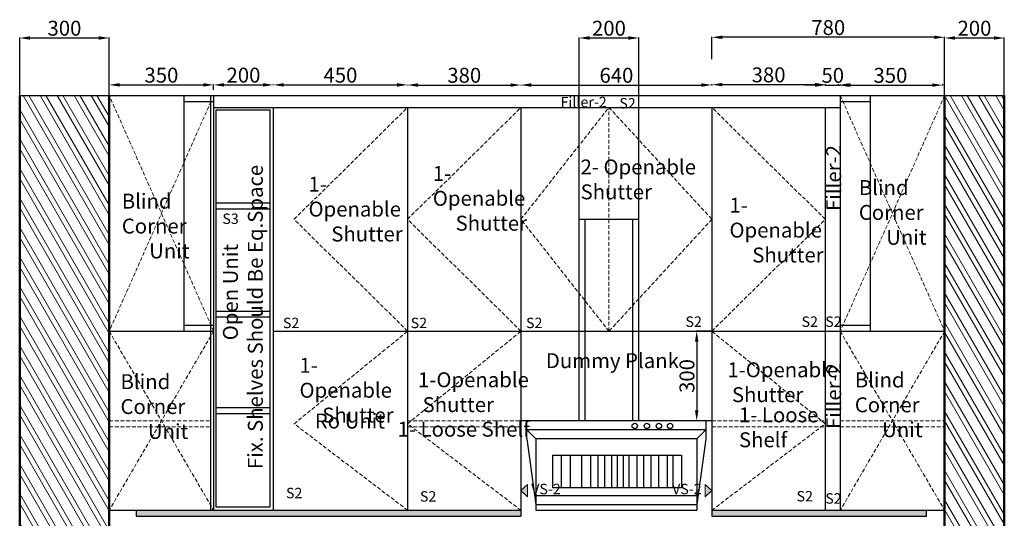
# Model space of a CAD drawing. Units: millimetres. Extents: x 407065 to 421840, y 1168257 to 1177792.
# Tile 13 of 17: x 412429 to 415729, y 1175560 to 1177230. Entities that reach past the tile are written whole.
import ezdxf

# ---------------------------------------------------------------- set-up
doc = ezdxf.new("R2010")
doc.units = ezdxf.units.MM
doc.linetypes.add('DASHED', pattern=[19.05, 12.7, -6.35])
for name, color, linetype, lineweight in [('A-ANNO-DIMS', 6, 'Continuous', 18), ('A-ANNO-SYMB', 6, 'Continuous', 18), ('A-ANNO-TEXT', 30, 'Continuous', 18), ('A-FURN', 3, 'Continuous', 25), ('A-FURN-HIDN', 7, 'DASHED', 18), ('A-FURN-PATT', 252, 'Continuous', 13), ('A-WALL', 7, 'Continuous', 50), ('A-WALL-PATT', 8, 'Continuous', 13)]:
    doc.layers.add(name, color=color, linetype=linetype, lineweight=lineweight)
doc.styles.get("Standard").update_dxf_attribs({"font": 'arial.ttf'})
doc.dimstyles.new('ISO-25', dxfattribs={"dimtxt": 50, "dimasz": 35, "dimexe": 1.25, "dimexo": 0.625, "dimtad": 1, "dimdec": 1, "dimtxsty": 'Standard', "dimcen": 35, "dimadec": 0, "dimazin": 0, "dimtfac": 1, "dimtdec": 1, "dimtmove": 0, "dimatfit": 3, "dimfxl": 1, "dimarcsym": 0})
pattern_1 = [(120, (-2714.86, -161.38), (-42.8942382, -24.765), []), (120, (-2708.816, -138.83), (-42.8942382, -24.765), [])]

# ---------------------------------------------------------------- blocks, each defined once
blk = doc.blocks.new('*D54')
at = {"layer": 'A-ANNO-DIMS', "color": 0, "lineweight": -2, "transparency": 16777216}
for p, q in [((412728.5, 1176995.6), (412728.5, 1177013)), ((412763.5, 1177011.8), (413043.5, 1177011.8)), ((413078.5, 1176995.6), (413078.5, 1177013))]:
    blk.add_line(p, q, dxfattribs=at)
at = {"layer": 'A-ANNO-DIMS', "color": 0, "transparency": 16777216}
for points in [[(412763.5, 1177017.6), (412763.5, 1177005.9), (412728.5, 1177011.8)], [(413043.5, 1177017.6), (413043.5, 1177005.9), (413078.5, 1177011.8)]]:
    blk.add_solid(points, dxfattribs=at)
at = {"layer": 'Defpoints', "color": 0, "transparency": 16777216}
for p in [(413078.5, 1177011.8), (412728.5, 1176995), (413078.5, 1176995)]:
    blk.add_point(p, dxfattribs=at)
at = {"layer": 'A-ANNO-DIMS', "color": 0, "transparency": 16777216, "insert": (412903.5, 1177037.9), "char_height": 50, "attachment_point": 5}
blk.add_mtext('350', dxfattribs=at)
blk = doc.blocks.new('*D55')
at = {"layer": 'A-ANNO-DIMS', "color": 0, "lineweight": -2, "transparency": 16777216}
for p, q in [((413078.5, 1177012.4), (413078.5, 1177013)), ((413113.5, 1177011.8), (413243.5, 1177011.8)), ((413278.5, 1177012.4), (413278.5, 1177013))]:
    blk.add_line(p, q, dxfattribs=at)
at = {"layer": 'A-ANNO-DIMS', "color": 0, "transparency": 16777216}
for points in [[(413113.5, 1177017.6), (413113.5, 1177005.9), (413078.5, 1177011.8)], [(413243.5, 1177017.6), (413243.5, 1177005.9), (413278.5, 1177011.8)]]:
    blk.add_solid(points, dxfattribs=at)
at = {"layer": 'Defpoints', "color": 0, "transparency": 16777216}
for p in [(413078.5, 1177011.8), (413278.5, 1177011.8), (413278.5, 1177011.8)]:
    blk.add_point(p, dxfattribs=at)
at = {"layer": 'A-ANNO-DIMS', "color": 0, "transparency": 16777216, "insert": (413178.5, 1177037.9), "char_height": 50, "attachment_point": 5}
blk.add_mtext('200', dxfattribs=at)
blk = doc.blocks.new('*D56')
at = {"layer": 'A-ANNO-DIMS', "color": 0, "lineweight": -2, "transparency": 16777216}
for p, q in [((413278.5, 1177012.1), (413278.5, 1177010.5)), ((413313.5, 1177011.8), (413693.5, 1177011.8)), ((413728.5, 1177012.1), (413728.5, 1177010.5))]:
    blk.add_line(p, q, dxfattribs=at)
at = {"layer": 'A-ANNO-DIMS', "color": 0, "transparency": 16777216}
for points in [[(413313.5, 1177017.6), (413313.5, 1177005.9), (413278.5, 1177011.8)], [(413693.5, 1177017.6), (413693.5, 1177005.9), (413728.5, 1177011.8)]]:
    blk.add_solid(points, dxfattribs=at)
at = {"layer": 'Defpoints', "color": 0, "transparency": 16777216}
for p in [(413278.5, 1177012.7), (413728.5, 1177012.7), (413728.5, 1177011.8)]:
    blk.add_point(p, dxfattribs=at)
at = {"layer": 'A-ANNO-DIMS', "color": 0, "transparency": 16777216, "insert": (413503.5, 1177037.9), "char_height": 50, "attachment_point": 5}
blk.add_mtext('450', dxfattribs=at)
blk = doc.blocks.new('*D57')
at = {"layer": 'A-ANNO-DIMS', "color": 0, "lineweight": -2, "transparency": 16777216}
for p, q in [((413728.5, 1177012.1), (413728.5, 1177010)), ((413763.5, 1177011.3), (414073.5, 1177011.3)), ((414108.5, 1177012.1), (414108.5, 1177010))]:
    blk.add_line(p, q, dxfattribs=at)
at = {"layer": 'A-ANNO-DIMS', "color": 0, "transparency": 16777216}
for points in [[(413763.5, 1177017.1), (413763.5, 1177005.4), (413728.5, 1177011.3)], [(414073.5, 1177017.1), (414073.5, 1177005.4), (414108.5, 1177011.3)]]:
    blk.add_solid(points, dxfattribs=at)
at = {"layer": 'Defpoints', "color": 0, "transparency": 16777216}
for p in [(413728.5, 1177012.7), (414108.5, 1177012.7), (414108.5, 1177011.3)]:
    blk.add_point(p, dxfattribs=at)
at = {"layer": 'A-ANNO-DIMS', "color": 0, "transparency": 16777216, "insert": (413918.5, 1177037.5), "char_height": 50, "attachment_point": 5}
blk.add_mtext('380', dxfattribs=at)
blk = doc.blocks.new('*D58')
at = {"layer": 'A-ANNO-DIMS', "color": 0, "lineweight": -2, "transparency": 16777216}
for p, q in [((414108.5, 1177012.1), (414108.5, 1177010)), ((414143.5, 1177011.3), (414713.5, 1177011.3)), ((414748.5, 1177012.1), (414748.5, 1177010))]:
    blk.add_line(p, q, dxfattribs=at)
at = {"layer": 'A-ANNO-DIMS', "color": 0, "transparency": 16777216}
for points in [[(414143.5, 1177017.1), (414143.5, 1177005.4), (414108.5, 1177011.3)], [(414713.5, 1177017.1), (414713.5, 1177005.4), (414748.5, 1177011.3)]]:
    blk.add_solid(points, dxfattribs=at)
at = {"layer": 'Defpoints', "color": 0, "transparency": 16777216}
for p in [(414108.5, 1177012.7), (414748.5, 1177012.7), (414748.5, 1177011.3)]:
    blk.add_point(p, dxfattribs=at)
at = {"layer": 'A-ANNO-DIMS', "color": 0, "transparency": 16777216, "insert": (414428.5, 1177037.4), "char_height": 50, "attachment_point": 5}
blk.add_mtext('640', dxfattribs=at)
blk = doc.blocks.new('*D59')
at = {"layer": 'A-ANNO-DIMS', "color": 0, "lineweight": -2, "transparency": 16777216}
for p, q in [((414748.5, 1177011.7), (414748.5, 1177013.9)), ((414783.5, 1177012.7), (415093.5, 1177012.7)), ((415128.5, 1177011.7), (415128.5, 1177013.9))]:
    blk.add_line(p, q, dxfattribs=at)
at = {"layer": 'A-ANNO-DIMS', "color": 0, "transparency": 16777216}
for points in [[(414783.5, 1177018.5), (414783.5, 1177006.9), (414748.5, 1177012.7)], [(415093.5, 1177018.5), (415093.5, 1177006.9), (415128.5, 1177012.7)]]:
    blk.add_solid(points, dxfattribs=at)
at = {"layer": 'Defpoints', "color": 0, "transparency": 16777216}
for p in [(414748.5, 1177011), (415128.5, 1177012.7), (415128.5, 1177011)]:
    blk.add_point(p, dxfattribs=at)
at = {"layer": 'A-ANNO-DIMS', "color": 0, "transparency": 16777216, "insert": (414938.5, 1177038.9), "char_height": 50, "attachment_point": 5}
blk.add_mtext('380', dxfattribs=at)
blk = doc.blocks.new('*D60')
at = {"layer": 'A-ANNO-DIMS', "color": 0, "lineweight": -2, "transparency": 16777216}
for p, q in [((415093.5, 1177011), (415058.5, 1177011)), ((415128.5, 1177013.3), (415128.5, 1177009.8)), ((415128.5, 1177011), (415178.5, 1177011)), ((415178.5, 1177013.3), (415178.5, 1177009.8)), ((415213.5, 1177011), (415248.5, 1177011))]:
    blk.add_line(p, q, dxfattribs=at)
at = {"layer": 'A-ANNO-DIMS', "color": 0, "transparency": 16777216}
for points in [[(415093.5, 1177016.9), (415093.5, 1177005.2), (415128.5, 1177011)], [(415213.5, 1177016.9), (415213.5, 1177005.2), (415178.5, 1177011)]]:
    blk.add_solid(points, dxfattribs=at)
at = {"layer": 'Defpoints', "color": 0, "transparency": 16777216}
for p in [(415128.5, 1177013.9), (415178.5, 1177013.9), (415178.5, 1177011)]:
    blk.add_point(p, dxfattribs=at)
at = {"layer": 'A-ANNO-DIMS', "color": 0, "transparency": 16777216, "insert": (415153.5, 1177037.2), "char_height": 50, "attachment_point": 5}
blk.add_mtext('50', dxfattribs=at)
blk = doc.blocks.new('*D61')
at = {"layer": 'A-ANNO-DIMS', "color": 0, "lineweight": -2, "transparency": 16777216}
for p, q in [((415171.8, 1177014.2), (415171.8, 1177009.8)), ((415206.8, 1177011), (415486.8, 1177011)), ((415521.8, 1177014.2), (415521.8, 1177009.8))]:
    blk.add_line(p, q, dxfattribs=at)
at = {"layer": 'A-ANNO-DIMS', "color": 0, "transparency": 16777216}
for points in [[(415206.8, 1177016.9), (415206.8, 1177005.2), (415171.8, 1177011)], [(415486.8, 1177016.9), (415486.8, 1177005.2), (415521.8, 1177011)]]:
    blk.add_solid(points, dxfattribs=at)
at = {"layer": 'Defpoints', "color": 0, "transparency": 16777216}
for p in [(415171.8, 1177014.8), (415521.8, 1177014.8), (415521.8, 1177011)]:
    blk.add_point(p, dxfattribs=at)
at = {"layer": 'A-ANNO-DIMS', "color": 0, "transparency": 16777216, "insert": (415346.8, 1177037.2), "char_height": 50, "attachment_point": 5}
blk.add_mtext('350', dxfattribs=at)
blk = doc.blocks.new('*D62')
at = {"layer": 'A-ANNO-DIMS', "color": 0, "lineweight": -2, "transparency": 16777216}
for p, q in [((414748.5, 1177098.3), (414748.5, 1177172.4)), ((415493.5, 1177171.2), (414783.5, 1177171.2)), ((415528.5, 1177098.3), (415528.5, 1177172.4))]:
    blk.add_line(p, q, dxfattribs=at)
at = {"layer": 'A-ANNO-DIMS', "color": 0, "transparency": 16777216}
for points in [[(414783.5, 1177177), (414783.5, 1177165.4), (414748.5, 1177171.2)], [(415493.5, 1177177), (415493.5, 1177165.4), (415528.5, 1177171.2)]]:
    blk.add_solid(points, dxfattribs=at)
at = {"layer": 'Defpoints', "color": 0, "transparency": 16777216}
for p in [(414748.5, 1177171.2), (414748.5, 1177097.6), (415528.5, 1177097.6)]:
    blk.add_point(p, dxfattribs=at)
at = {"layer": 'A-ANNO-DIMS', "color": 0, "transparency": 16777216, "insert": (415138.5, 1177197.4), "char_height": 50, "attachment_point": 5}
blk.add_mtext('780', dxfattribs=at)
blk = doc.blocks.new('*D81')
at = {"layer": 'A-ANNO-DIMS', "color": 0, "lineweight": -2, "transparency": 16777216}
for p, q in [((414747.9, 1176186.4), (414696.2, 1176186.4)), ((414697.5, 1176151.4), (414697.5, 1175921.4)), ((414747.9, 1175886.4), (414696.2, 1175886.4))]:
    blk.add_line(p, q, dxfattribs=at)
at = {"layer": 'A-ANNO-DIMS', "color": 0, "transparency": 16777216}
for points in [[(414691.7, 1176151.4), (414703.3, 1176151.4), (414697.5, 1176186.4)], [(414691.7, 1175921.4), (414703.3, 1175921.4), (414697.5, 1175886.4)]]:
    blk.add_solid(points, dxfattribs=at)
at = {"layer": 'Defpoints', "color": 0, "transparency": 16777216}
for p in [(414748.5, 1176186.4), (414697.5, 1175886.4), (414748.5, 1175886.4)]:
    blk.add_point(p, dxfattribs=at)
at = {"layer": 'A-ANNO-DIMS', "color": 0, "transparency": 16777216, "insert": (414671.3, 1176036.4), "char_height": 50, "attachment_point": 5, "rotation": 90}
blk.add_mtext('300', dxfattribs=at)
blk = doc.blocks.new('*D194')
at = {"layer": 'A-ANNO-DIMS', "color": 0, "lineweight": -2, "transparency": 16777216}
for p, q in [((412428.5, 1176977), (412428.5, 1177170.2)), ((412463.5, 1177168.9), (412693.5, 1177168.9)), ((412728.5, 1176977), (412728.5, 1177170.2))]:
    blk.add_line(p, q, dxfattribs=at)
at = {"layer": 'A-ANNO-DIMS', "color": 0, "transparency": 16777216}
for points in [[(412463.5, 1177174.7), (412463.5, 1177163.1), (412428.5, 1177168.9)], [(412693.5, 1177174.7), (412693.5, 1177163.1), (412728.5, 1177168.9)]]:
    blk.add_solid(points, dxfattribs=at)
at = {"layer": 'Defpoints', "color": 0, "transparency": 16777216}
for p in [(412728.5, 1177168.9), (412428.5, 1176976.4), (412728.5, 1176976.4)]:
    blk.add_point(p, dxfattribs=at)
at = {"layer": 'A-ANNO-DIMS', "color": 0, "transparency": 16777216, "insert": (412578.5, 1177195.1), "char_height": 50, "attachment_point": 5}
blk.add_mtext('300', dxfattribs=at)
blk = doc.blocks.new('*D195')
at = {"layer": 'A-ANNO-DIMS', "color": 0, "lineweight": -2, "transparency": 16777216}
for p, q in [((415528.5, 1176977), (415528.5, 1177170.2)), ((415563.5, 1177168.9), (415693.5, 1177168.9)), ((415728.5, 1176977), (415728.5, 1177170.2))]:
    blk.add_line(p, q, dxfattribs=at)
at = {"layer": 'A-ANNO-DIMS', "color": 0, "transparency": 16777216}
for points in [[(415563.5, 1177174.7), (415563.5, 1177163.1), (415528.5, 1177168.9)], [(415693.5, 1177174.7), (415693.5, 1177163.1), (415728.5, 1177168.9)]]:
    blk.add_solid(points, dxfattribs=at)
at = {"layer": 'Defpoints', "color": 0, "transparency": 16777216}
for p in [(415728.5, 1177168.9), (415528.5, 1176976.4), (415728.5, 1176976.4)]:
    blk.add_point(p, dxfattribs=at)
at = {"layer": 'A-ANNO-DIMS', "color": 0, "transparency": 16777216, "insert": (415628.5, 1177195.1), "char_height": 50, "attachment_point": 5}
blk.add_mtext('200', dxfattribs=at)
blk = doc.blocks.new('*D196')
at = {"layer": 'A-ANNO-DIMS', "color": 0, "lineweight": -2, "transparency": 16777216}
for p, q in [((414303.5, 1176562), (414303.5, 1177170.2)), ((414338.5, 1177168.9), (414468.5, 1177168.9)), ((414503.5, 1176562), (414503.5, 1177170.2))]:
    blk.add_line(p, q, dxfattribs=at)
at = {"layer": 'A-ANNO-DIMS', "color": 0, "transparency": 16777216}
for points in [[(414338.5, 1177174.7), (414338.5, 1177163.1), (414303.5, 1177168.9)], [(414468.5, 1177174.7), (414468.5, 1177163.1), (414503.5, 1177168.9)]]:
    blk.add_solid(points, dxfattribs=at)
at = {"layer": 'Defpoints', "color": 0, "transparency": 16777216}
for p in [(414503.5, 1177168.9), (414303.5, 1176561.4), (414503.5, 1176561.4)]:
    blk.add_point(p, dxfattribs=at)
at = {"layer": 'A-ANNO-DIMS', "color": 0, "transparency": 16777216, "insert": (414403.5, 1177195.1), "char_height": 50, "attachment_point": 5}
blk.add_mtext('200', dxfattribs=at)

msp = doc.modelspace()

# ---------------------------------------------------------------- hatches: boundary and pattern name
at = {"layer": 'A-FURN'}
h = msp.add_hatch(color=256, dxfattribs=at)
h.dxf.hatch_style = 1
h.paths.add_polyline_path([(414130.6789, 1175673.0906), (414108.5012, 1175652.4221), (414130.6789, 1175631.7537)])
h = msp.add_hatch(color=256, dxfattribs=at)
h.dxf.hatch_style = 1
h.paths.add_polyline_path([(414726.3235, 1175673.0906), (414726.3235, 1175631.7537), (414748.5012, 1175652.4221)])
at = {"layer": 'A-FURN-PATT'}
h = msp.add_hatch(color=256, dxfattribs=at)
h.dxf.hatch_style = 1
h.paths.add_polyline_path([(414108.5012, 1175586.413), (412818.3307, 1175586.413), (412818.3307, 1175566.413), (414108.5012, 1175566.413)])
h = msp.add_hatch(color=256, dxfattribs=at)
h.dxf.hatch_style = 1
h.paths.add_polyline_path([(415468.2273, 1175586.413), (414748.5012, 1175586.413), (414748.5012, 1175566.413), (415468.2273, 1175566.413)])
at = {"layer": 'A-WALL-PATT'}
h = msp.add_hatch(dxfattribs=at)
h.set_pattern_fill('ANSI32', color=256, scale=5.2, angle=75)
h.set_pattern_definition(pattern_1)
h.paths.add_polyline_path([(412728.5012, 1176976.413), (412428.5012, 1176976.413), (412428.5012, 1174126.413), (412728.5012, 1174126.413)])
h = msp.add_hatch(dxfattribs=at)
h.set_pattern_fill('ANSI32', color=256, scale=5.2, angle=75)
h.set_pattern_definition(pattern_1)
h.paths.add_polyline_path([(415728.5012, 1176976.413), (415528.5012, 1176976.413), (415528.5012, 1174126.413), (415728.5012, 1174126.413)])

# ---------------------------------------------------------------- linework, layer by layer
at = {"layer": 'A-ANNO-SYMB'}
for points in [[(414130.6789, 1175673.0906), (414108.5012, 1175652.4221), (414130.6789, 1175631.7537)], [(414726.3235, 1175673.0906), (414748.5012, 1175652.4221), (414726.3235, 1175631.7537)]]:
    msp.add_lwpolyline(points, close=True, dxfattribs=at)
at = {"layer": 'A-FURN'}
for p, q in [((412428.5012, 1176976.413), (415728.5012, 1176976.413)), ((412978.5012, 1176976.413), (412978.5012, 1176186.413)), ((412978.5012, 1176956.413), (413078.5012, 1176956.413)), ((413068.5012, 1176976.413), (413068.5012, 1175586.413)), ((413078.5012, 1176976.413), (413078.5012, 1175586.413)), ((415178.5012, 1176976.413), (415178.5012, 1175586.413)), ((415178.5012, 1176956.413), (415278.5012, 1176956.413)), ((415278.5012, 1176976.413), (415278.5012, 1176186.413)), ((413078.5012, 1176936.413), (415178.5012, 1176936.413)), ((413278.5012, 1176936.413), (413278.5012, 1175586.413)), ((413728.5012, 1176936.413), (413728.5012, 1175586.413)), ((414108.5012, 1176936.413), (414108.5012, 1175566.413)), ((414748.5012, 1176936.413), (414748.5012, 1175566.413)), ((415128.5012, 1176936.413), (415128.5012, 1175586.413)), ((413266.6662, 1176615.3867), (413087.0747, 1176615.3867)), ((413266.6662, 1176595.3867), (413087.0747, 1176595.3867)), ((414303.5012, 1175886.413), (414303.5012, 1176561.413)), ((414303.5012, 1176561.413), (414503.5012, 1176561.413)), ((414323.5012, 1175886.413), (414323.5012, 1176561.413)), ((414483.5012, 1175886.413), (414483.5012, 1176561.413)), ((414503.5012, 1175886.413), (414503.5012, 1176561.413)), ((413266.6662, 1176253.0057), (413087.0747, 1176253.0057)), ((413266.6662, 1176233.0057), (413087.0747, 1176233.0057)), ((412728.5012, 1176186.413), (413078.5012, 1176186.413)), ((412978.5012, 1176206.413), (413078.5012, 1176206.413)), ((413278.5012, 1176186.413), (415528.5012, 1176186.413)), ((415178.5012, 1176206.413), (415278.5012, 1176206.413)), ((413266.6662, 1175929.8197), (413087.0747, 1175929.8197)), ((413266.6662, 1175909.8197), (413087.0747, 1175909.8197)), ((414748.5012, 1175886.413), (414108.5012, 1175886.413)), ((414128.5012, 1175826.413), (414128.5012, 1175886.413)), ((414728.5012, 1175856.413), (414128.5012, 1175856.413)), ((414128.5012, 1175856.413), (414158.5012, 1175826.413)), ((414728.5012, 1175856.413), (414698.5012, 1175826.413)), ((414728.5012, 1175886.413), (414728.5012, 1175826.413)), ((414128.5012, 1175826.413), (414158.5012, 1175606.413)), ((414698.5012, 1175826.413), (414158.5012, 1175826.413)), ((414158.5012, 1175826.413), (414158.5012, 1175586.413)), ((414728.5012, 1175826.413), (414698.5012, 1175606.413)), ((414698.5012, 1175826.413), (414698.5012, 1175586.413)), ((414242.9928, 1175770.6517), (414242.9928, 1175662.0889)), ((414273.6739, 1175770.6517), (414273.6739, 1175662.0889)), ((414311.7778, 1175770.6517), (414311.7778, 1175662.0889)), ((414341.9639, 1175770.6517), (414341.9639, 1175662.0889)), ((414366.2118, 1175770.6517), (414366.2118, 1175662.0889)), ((414388.9751, 1175770.6517), (414388.9751, 1175662.0889)), ((414412.2333, 1175770.6517), (414412.2333, 1175662.0889)), ((414431.2259, 1175770.6517), (414431.2259, 1175662.0889)), ((414451.3269, 1175770.6517), (414451.3269, 1175662.0889)), ((414470.6262, 1175770.6517), (414470.6262, 1175662.0889)), ((414496.3587, 1175770.6517), (414496.3587, 1175662.0889)), ((414519.122, 1175770.6517), (414519.122, 1175662.0889)), ((414543.3699, 1175770.6517), (414543.3699, 1175662.0889)), ((414569.5973, 1175770.6517), (414569.5973, 1175662.0889)), ((414598.7937, 1175770.6517), (414598.7937, 1175662.0889)), ((414618.0931, 1175770.6517), (414618.0931, 1175662.0889)), ((414158.5012, 1175636.413), (414698.5012, 1175636.413)), ((414158.5012, 1175606.413), (414698.5012, 1175606.413)), ((412728.5012, 1175586.413), (414108.5012, 1175586.413)), ((412818.3307, 1175586.413), (412818.3307, 1175566.413)), ((412818.3307, 1175566.413), (414108.5012, 1175566.413)), ((414158.5012, 1175586.413), (414698.5012, 1175586.413)), ((414748.5012, 1175586.413), (415528.5012, 1175586.413)), ((414748.5012, 1175566.413), (415468.2273, 1175566.413)), ((415468.2273, 1175566.413), (415468.2273, 1175586.413))]:
    msp.add_line(p, q, dxfattribs=at)
for points in [[(413087.0747, 1176928.6875), (413266.6662, 1176928.6875), (413266.6662, 1175597.5096), (413087.0747, 1175597.5096)], [(414215.4815, 1175770.6517), (414646.9703, 1175770.6517), (414646.9703, 1175662.0889), (414215.4815, 1175662.0889)]]:
    msp.add_lwpolyline(points, close=True, dxfattribs=at)
for centre in [(414490.0655, 1175869.1558), (414530.6257, 1175869.1558), (414570.849, 1175869.1558), (414608.3798, 1175869.1558)]:
    msp.add_circle(centre, 9.0999, dxfattribs=at)
at = {"layer": 'A-FURN-HIDN'}
for p, q in [((413078.5012, 1176186.413), (412728.5012, 1176976.413)), ((413069.6404, 1176956.413), (412728.5012, 1176186.413)), ((415178.5012, 1176976.413), (415528.5012, 1176186.413)), ((415528.5012, 1176976.413), (415178.5012, 1176186.413)), ((414108.5012, 1176561.413), (414403.5012, 1176936.413)), ((414403.5012, 1176186.413), (414403.5012, 1176936.413)), ((414403.5012, 1176936.413), (414748.5012, 1176561.413)), ((414403.5012, 1176186.413), (414108.5012, 1176561.413)), ((414748.5012, 1176561.413), (414403.5012, 1176186.413)), ((412728.5012, 1176186.413), (413078.5012, 1175586.413)), ((413078.5012, 1176186.413), (412728.5012, 1175586.413)), ((415178.5012, 1176186.413), (415528.5012, 1175586.413)), ((415528.5012, 1176186.413), (415178.5012, 1175586.413)), ((412728.5012, 1175886.413), (413068.5012, 1175886.413)), ((412728.5012, 1175866.413), (413068.5012, 1175866.413)), ((413728.5012, 1175886.413), (414108.5012, 1175886.413)), ((413728.5012, 1175866.413), (414108.5012, 1175866.413)), ((414748.5012, 1175886.413), (415128.5012, 1175886.413)), ((414748.5012, 1175866.413), (415128.5012, 1175866.413)), ((415178.5012, 1175886.413), (415528.5012, 1175886.413)), ((415178.5012, 1175866.413), (415528.5012, 1175866.413))]:
    msp.add_line(p, q, dxfattribs=at)
for points in [[(413728.5012, 1175586.413), (413348.5012, 1175876.413), (413728.5012, 1176186.413), (413348.5012, 1176561.413), (413728.5012, 1176936.413)], [(414108.5012, 1175586.413), (413728.5012, 1175876.413), (414108.5012, 1176186.413), (413728.5012, 1176561.413), (414108.5012, 1176936.413)], [(414748.5012, 1175586.413), (415128.5012, 1175876.413), (414748.5012, 1176186.413), (415128.5012, 1176561.413), (414748.5012, 1176936.413)]]:
    msp.add_lwpolyline(points, dxfattribs=at)
at = {"layer": 'A-WALL'}
for p, q in [((412428.5012, 1176976.413), (412428.5012, 1174126.413)), ((412728.5012, 1176976.413), (412728.5012, 1174126.413)), ((415528.5012, 1176976.413), (415528.5012, 1174126.413)), ((415728.5012, 1176976.413), (415728.5012, 1174126.413))]:
    msp.add_line(p, q, dxfattribs=at)

# ---------------------------------------------------------------- texts
at = {"layer": 'A-ANNO-TEXT'}
for s, width, insert, char_height, attachment_point in [('     Filler-2', 382.409863, (414187.8475, 1176971.7278), 35, 1), ('S2', 382.409863, (414438.1888, 1176967.6805), 35, 1), ('2- Openable Shutter', 467.834353, (414308.353, 1176761.764), 50, 1), ('1- Openable\\P     Shutter', 382.409863, (413813.0953, 1176740.0419), 50, 1), ('1- Openable\\P     Shutter', 382.409863, (413396.487, 1176703.9152), 50, 1), ('Blind Corner\\P      Unit', 382.409863, (415240.898, 1176692.8107), 50, 1), ('Blind Corner\\P      Unit', 382.409863, (412770.672, 1176647.1576), 50, 1), ('1- Openable\\P     Shutter', 382.409863, (414807.3356, 1176633.5179), 50, 1), ('S3', 382.409863, (413107.7197, 1176580.7009), 35, 1), ('S2', 382.409863, (413310.7196, 1176231.7181), 35, 1), ('S2', 382.409863, (413738.915, 1176231.7181), 35, 1), ('S2', 382.409863, (414125.4154, 1176231.7181), 35, 1), ('S2', 382.409863, (414659.8885, 1176235.9389), 35, 1), ('S2', 382.409863, (415048.8999, 1176235.9863), 35, 1), ('S2', 382.409863, (415128.5012, 1176235.9863), 35, 1), ('1- Openable\\P     Shutter', 382.409863, (413366.229, 1176097.0939), 50, 1), ('Dummy Plank', 510.114273, (414192.0951, 1176112.8019), 50, 1), ('     1-Openable\\P      Shutter', 520.083559, (414723.9737, 1176082.1969), 50, 1), ('Blind Corner\\P      Unit', 382.409863, (412766.3782, 1176042.3897), 50, 1), ('     1-Openable\\P      Shutter', 520.083559, (413687.1676, 1176048.7697), 50, 1), ('Blind Corner\\P      Unit', 382.409863, (415227.4042, 1176048.2259), 50, 1), ('1- Loose Shelf', 382.409863, (414839.2513, 1175931.0727), 50, 1), ('      Ro Unit', 382.409863, (413325.9536, 1175910.5532), 50, 1), ('1- Loose Shelf', 502.711169, (413695.2644, 1175883.1479), 50, 1), ('S2', 382.409863, (413321.0208, 1175661.7419), 35, 1), ('VS-2', 382.409863, (414241.8674, 1175675.2261), 35, 3), ('VS-2', 382.409863, (414615.135, 1175675.2261), 35, 1), ('S2', 382.409863, (413769.9307, 1175650.5444), 35, 1), ('S2', 382.409863, (415032.0763, 1175651.0661), 35, 1), ('S2', 382.409863, (415128.5012, 1175643.6972), 35, 1)]:
    msp.add_mtext_dynamic_manual_height_columns(s, width=width, gutter_width=12.5, heights=[0], dxfattribs=dict(at, insert=insert, char_height=char_height, attachment_point=attachment_point))
at = {"layer": 'A-ANNO-TEXT', "char_height": 50, "attachment_point": 1, "rotation": 90}
for s, width, insert in [('     Filler-2', 382.409863, (415131.4515, 1176512.8254)), ('Fix. Shelves Should Be Eq.Space', 1098.753437, (413193.3449, 1175724.4097)), ('    Open Unit', 468.025593, (413109.7442, 1176094.9095)), ('     Filler-2', 382.409863, (415131.4515, 1175782.4118))]:
    msp.add_mtext_dynamic_manual_height_columns(s, width=width, gutter_width=12.5, heights=[0], dxfattribs=dict(at, insert=insert))

# ---------------------------------------------------------------- dimensions: what is measured, and where the dimension line sits
at = {"layer": 'A-ANNO-DIMS'}
for base, p1, p2, override, picture, middle in [((412728.5012, 1177168.913), (412428.5012, 1176976.413), (412728.5012, 1176976.413), {"dimdec": 0, "dimlfac": 1, "dimrnd": 0, "dimzin": 0, "dimdsep": 46, "dimlunit": 2}, '*D194', (412578.5012, 1177195.0837)), ((414503.5012, 1177168.913), (414303.5012, 1176561.413), (414503.5012, 1176561.413), {"dimdec": 0, "dimlfac": 1, "dimrnd": 0, "dimzin": 0, "dimdsep": 46, "dimlunit": 2}, '*D196', (414403.5012, 1177195.0667)), ((414748.5012, 1177171.1988), (415528.5012, 1177097.6488), (414748.5012, 1177097.6488), {"dimclrd": 0, "dimclre": 0, "dimclrt": 0}, '*D62', (415138.5012, 1177197.3525)), ((415728.5012, 1177168.913), (415528.5012, 1176976.413), (415728.5012, 1176976.413), {"dimdec": 0, "dimlfac": 1, "dimrnd": 0, "dimzin": 0, "dimdsep": 46, "dimlunit": 2}, '*D195', (415628.5012, 1177195.0667)), ((413078.5012, 1177011.7502), (412728.5012, 1176995.0191), (413078.5012, 1176995.0191), {"dimclrd": 0, "dimclre": 0, "dimclrt": 0}, '*D54', (412903.5012, 1177037.9209)), ((413278.5012, 1177011.7502), (413078.5012, 1177011.7502), (413278.5012, 1177011.7502), {"dimclrd": 0, "dimclre": 0, "dimclrt": 0}, '*D55', (413178.5012, 1177037.9038)), ((413728.5012, 1177011.7502), (413278.5012, 1177012.6877), (413728.5012, 1177012.6877), {"dimclrd": 0, "dimclre": 0, "dimclrt": 0}, '*D56', (413503.5012, 1177037.9038)), ((414108.5012, 1177011.2814), (413728.5012, 1177012.6877), (414108.5012, 1177012.6877), {"dimclrd": 0, "dimclre": 0, "dimclrt": 0}, '*D57', (413918.5012, 1177037.4521)), ((414748.5012, 1177011.2814), (414108.5012, 1177012.6877), (414748.5012, 1177012.6877), {"dimclrd": 0, "dimclre": 0, "dimclrt": 0}, '*D58', (414428.5012, 1177037.4351)), ((415128.5012, 1177012.6877), (414748.5012, 1177011.047), (415128.5012, 1177011.047), {"dimclrd": 0, "dimclre": 0, "dimclrt": 0}, '*D59', (414938.5012, 1177038.8584)), ((415521.848, 1177011.047), (415171.848, 1177014.797), (415521.848, 1177014.797), {"dimclrd": 0, "dimclre": 0, "dimclrt": 0}, '*D61', (415346.848, 1177037.2177))]:
    dim = msp.add_linear_dim(base=base, p1=p1, p2=p2, dimstyle='ISO-25', override=override, dxfattribs=at)
    dim.commit()
    dim.dimension.update_dxf_attribs({"geometry": picture, "text_midpoint": middle})
dim = msp.add_linear_dim(base=(415178.5012, 1177011.047), p1=(415128.5012, 1177013.9377), p2=(415178.5012, 1177013.9377), dimstyle='ISO-25', override={"dimclrd": 0, "dimclre": 0, "dimclrt": 0}, dxfattribs=at)
dim.commit()
dim.dimension.update_dxf_attribs({"geometry": '*D60', "text_midpoint": (415153.5012, 1177011.047), "dimtype": 160})
dim = msp.add_linear_dim(base=(414697.4904, 1175886.413), p1=(414748.5012, 1176186.413), p2=(414748.5012, 1175886.413), angle=90, dimstyle='ISO-25', override={"dimclrd": 0, "dimclre": 0, "dimclrt": 0}, dxfattribs=at)
dim.commit()
dim.dimension.update_dxf_attribs({"geometry": '*D81', "text_midpoint": (414671.3197, 1176036.413)})

doc.saveas('drawing.dxf')
